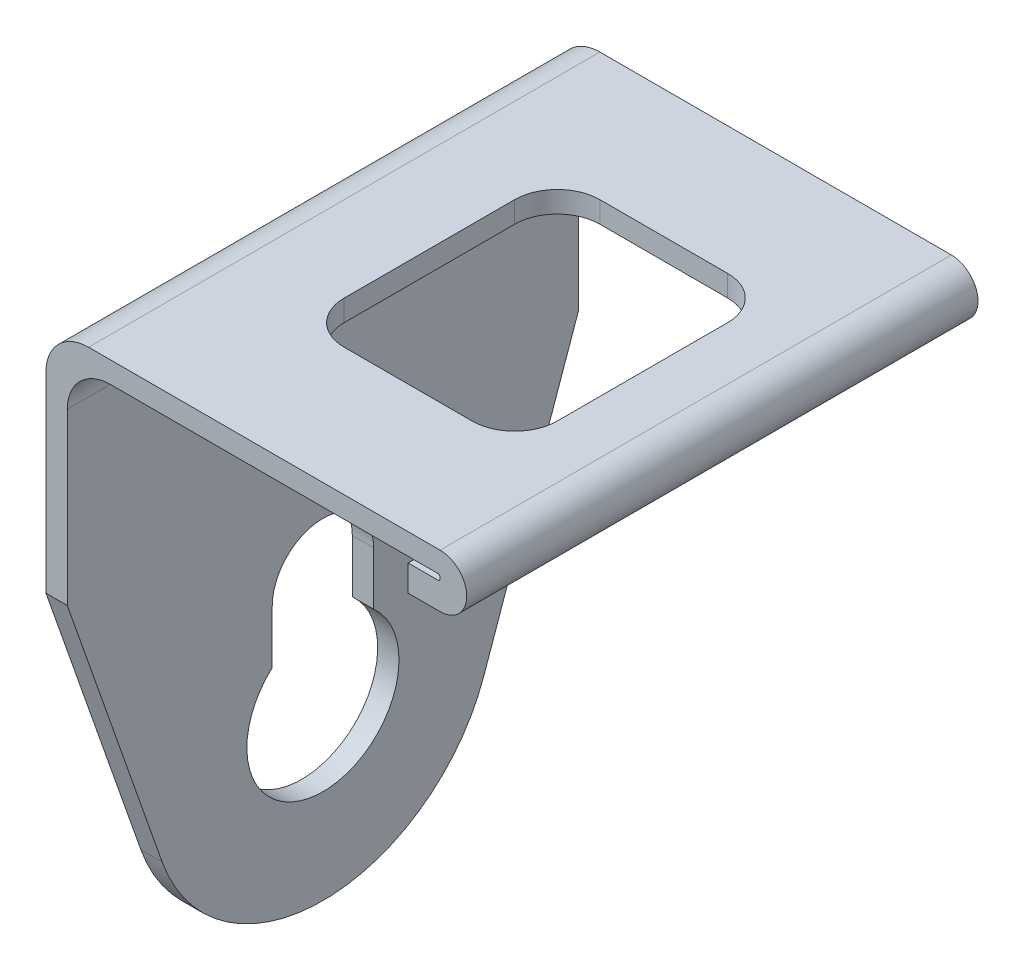
ISO-10303-21;
HEADER;
FILE_DESCRIPTION(('STEP AP214'),'2;1');
FILE_NAME('part.step','',(''),(''),'','','');
FILE_SCHEMA(('AUTOMOTIVE_DESIGN { 1 0 10303 214 1 1 1 1 }'));
ENDSEC;
DATA;
#1=APPLICATION_CONTEXT('core data for automotive mechanical design processes');
#2=APPLICATION_PROTOCOL_DEFINITION('international standard','automotive_design',2000,#1);
#3=PRODUCT_CONTEXT('',#1,'mechanical');
#4=PRODUCT('Part','Part','',(#3));
#5=PRODUCT_RELATED_PRODUCT_CATEGORY('part','',(#4));
#6=PRODUCT_DEFINITION_FORMATION('','',#4);
#7=PRODUCT_DEFINITION_CONTEXT('part definition',#1,'design');
#8=PRODUCT_DEFINITION('design','',#6,#7);
#9=PRODUCT_DEFINITION_SHAPE('','',#8);
#10=(LENGTH_UNIT() NAMED_UNIT(*) SI_UNIT(.MILLI.,.METRE.));
#11=(NAMED_UNIT(*) PLANE_ANGLE_UNIT() SI_UNIT($,.RADIAN.));
#12=(NAMED_UNIT(*) SI_UNIT($,.STERADIAN.) SOLID_ANGLE_UNIT());
#13=UNCERTAINTY_MEASURE_WITH_UNIT(LENGTH_MEASURE(1.E-05),#10,'distance_accuracy_value','');
#14=(GEOMETRIC_REPRESENTATION_CONTEXT(3) GLOBAL_UNCERTAINTY_ASSIGNED_CONTEXT((#13)) GLOBAL_UNIT_ASSIGNED_CONTEXT((#10,
#11,#12)) REPRESENTATION_CONTEXT('',''));
#15=CARTESIAN_POINT('',(0.,0.,0.));
#16=DIRECTION('',(0.,0.,1.));
#17=DIRECTION('',(1.,0.,0.));
#18=AXIS2_PLACEMENT_3D('',#15,#16,#17);
#19=CARTESIAN_POINT('',(0.,-2.,12.));
#20=DIRECTION('',(1.,0.,0.));
#21=DIRECTION('',(0.,1.,0.));
#22=AXIS2_PLACEMENT_3D('',#19,#20,#21);
#23=PLANE('',#22);
#24=DIRECTION('',(0.,1.,0.));
#25=VECTOR('',#24,1.);
#26=CARTESIAN_POINT('',(0.,-2.,-2.38));
#27=LINE('',#26,#25);
#28=CARTESIAN_POINT('',(0.,-18.3390791067752,-2.38));
#29=VERTEX_POINT('',#28);
#30=CARTESIAN_POINT('',(0.,-15.84,-2.38));
#31=VERTEX_POINT('',#30);
#32=EDGE_CURVE('E242',#29,#31,#27,.T.);
#33=ORIENTED_EDGE('',*,*,#32,.T.);
#34=CARTESIAN_POINT('',(0.,-15.84,0.));
#35=DIRECTION('',(1.,0.,0.));
#36=DIRECTION('',(0.,1.,0.));
#37=AXIS2_PLACEMENT_3D('',#34,#35,#36);
#38=CIRCLE('',#37,2.38);
#39=CARTESIAN_POINT('',(0.,-15.84,2.38));
#40=VERTEX_POINT('',#39);
#41=EDGE_CURVE('E245',#31,#40,#38,.T.);
#42=ORIENTED_EDGE('',*,*,#41,.T.);
#43=DIRECTION('',(0.,-1.,0.));
#44=VECTOR('',#43,1.);
#45=CARTESIAN_POINT('',(0.,-2.,2.38));
#46=LINE('',#45,#44);
#47=CARTESIAN_POINT('',(0.,-18.3390791067752,2.38));
#48=VERTEX_POINT('',#47);
#49=EDGE_CURVE('E240',#40,#48,#46,.T.);
#50=ORIENTED_EDGE('',*,*,#49,.T.);
#51=CARTESIAN_POINT('',(0.,-21.,0.));
#52=DIRECTION('',(1.,0.,0.));
#53=DIRECTION('',(0.,1.,0.));
#54=AXIS2_PLACEMENT_3D('',#51,#52,#53);
#55=CIRCLE('',#54,3.57);
#56=EDGE_CURVE('E220',#48,#29,#55,.T.);
#57=ORIENTED_EDGE('',*,*,#56,.T.);
#58=EDGE_LOOP('',(#33,#42,#50,#57));
#59=FACE_BOUND('',#58,.T.);
#60=CARTESIAN_POINT('',(0.,-21.,0.));
#61=DIRECTION('',(1.,0.,0.));
#62=DIRECTION('',(0.,1.,0.));
#63=AXIS2_PLACEMENT_3D('',#60,#61,#62);
#64=CIRCLE('',#63,7.99999999999971);
#65=CARTESIAN_POINT('',(0.,-23.655635881311,7.54636323442549));
#66=VERTEX_POINT('',#65);
#67=CARTESIAN_POINT('',(0.,-23.655635881311,-7.54636323442549));
#68=VERTEX_POINT('',#67);
#69=EDGE_CURVE('E268',#66,#68,#64,.T.);
#70=ORIENTED_EDGE('',*,*,#69,.F.);
#71=DIRECTION('',(0.,-0.943295404303216,-0.331954485163903));
#72=VECTOR('',#71,1.);
#73=CARTESIAN_POINT('',(0.,-2.99174402198394,14.8181802626367));
#74=LINE('',#73,#72);
#75=CARTESIAN_POINT('',(0.,-11.0000000000005,12.));
#76=VERTEX_POINT('',#75);
#77=EDGE_CURVE('E255',#76,#66,#74,.T.);
#78=ORIENTED_EDGE('',*,*,#77,.F.);
#79=DIRECTION('',(0.,-1.,0.));
#80=VECTOR('',#79,1.);
#81=CARTESIAN_POINT('',(0.,-2.,12.));
#82=LINE('',#81,#80);
#83=CARTESIAN_POINT('',(0.,-2.,12.));
#84=VERTEX_POINT('',#83);
#85=EDGE_CURVE('E329',#84,#76,#82,.T.);
#86=ORIENTED_EDGE('',*,*,#85,.F.);
#87=DIRECTION('',(0.,0.,-1.));
#88=VECTOR('',#87,1.);
#89=CARTESIAN_POINT('',(0.,-2.,12.));
#90=LINE('',#89,#88);
#91=CARTESIAN_POINT('',(0.,-2.,-12.));
#92=VERTEX_POINT('',#91);
#93=EDGE_CURVE('E379',#84,#92,#90,.T.);
#94=ORIENTED_EDGE('',*,*,#93,.T.);
#95=DIRECTION('',(0.,-1.,0.));
#96=VECTOR('',#95,1.);
#97=CARTESIAN_POINT('',(0.,-2.,-12.));
#98=LINE('',#97,#96);
#99=CARTESIAN_POINT('',(0.,-11.0000000000005,-12.));
#100=VERTEX_POINT('',#99);
#101=EDGE_CURVE('E353',#92,#100,#98,.T.);
#102=ORIENTED_EDGE('',*,*,#101,.T.);
#103=DIRECTION('',(0.,-0.943295404303216,0.331954485163903));
#104=VECTOR('',#103,1.);
#105=CARTESIAN_POINT('',(0.,-10.5068913890147,-12.1735295373463));
#106=LINE('',#105,#104);
#107=EDGE_CURVE('E264',#100,#68,#106,.T.);
#108=ORIENTED_EDGE('',*,*,#107,.T.);
#109=EDGE_LOOP('',(#70,#78,#86,#94,#102,#108));
#110=FACE_BOUND('',#109,.T.);
#111=ADVANCED_FACE('F39',(#59,#110),#23,.F.);
#112=CARTESIAN_POINT('',(1.,-29.,12.));
#113=DIRECTION('',(-1.,0.,0.));
#114=DIRECTION('',(0.,-1.,0.));
#115=AXIS2_PLACEMENT_3D('',#112,#113,#114);
#116=PLANE('',#115);
#117=DIRECTION('',(0.,-1.,0.));
#118=VECTOR('',#117,1.);
#119=CARTESIAN_POINT('',(1.,-15.84,2.38));
#120=LINE('',#119,#118);
#121=CARTESIAN_POINT('',(1.,-15.84,2.38));
#122=VERTEX_POINT('',#121);
#123=CARTESIAN_POINT('',(1.,-18.3390791067752,2.38));
#124=VERTEX_POINT('',#123);
#125=EDGE_CURVE('E224',#122,#124,#120,.T.);
#126=ORIENTED_EDGE('',*,*,#125,.F.);
#127=CARTESIAN_POINT('',(1.,-15.84,0.));
#128=DIRECTION('',(1.,0.,0.));
#129=DIRECTION('',(0.,1.,0.));
#130=AXIS2_PLACEMENT_3D('',#127,#128,#129);
#131=CIRCLE('',#130,2.38);
#132=CARTESIAN_POINT('',(1.,-15.84,-2.38));
#133=VERTEX_POINT('',#132);
#134=EDGE_CURVE('E62',#133,#122,#131,.T.);
#135=ORIENTED_EDGE('',*,*,#134,.F.);
#136=DIRECTION('',(0.,1.,0.));
#137=VECTOR('',#136,1.);
#138=CARTESIAN_POINT('',(1.,-15.84,-2.38));
#139=LINE('',#138,#137);
#140=CARTESIAN_POINT('',(1.,-18.3390791067752,-2.38));
#141=VERTEX_POINT('',#140);
#142=EDGE_CURVE('E230',#141,#133,#139,.T.);
#143=ORIENTED_EDGE('',*,*,#142,.F.);
#144=CARTESIAN_POINT('',(1.,-21.,0.));
#145=DIRECTION('',(1.,0.,0.));
#146=DIRECTION('',(0.,1.,0.));
#147=AXIS2_PLACEMENT_3D('',#144,#145,#146);
#148=CIRCLE('',#147,3.57);
#149=EDGE_CURVE('E212',#124,#141,#148,.T.);
#150=ORIENTED_EDGE('',*,*,#149,.F.);
#151=EDGE_LOOP('',(#126,#135,#143,#150));
#152=FACE_BOUND('',#151,.T.);
#153=DIRECTION('',(0.,-0.943295404303216,-0.331954485163903));
#154=VECTOR('',#153,1.);
#155=CARTESIAN_POINT('',(1.,-4.96970526594021,14.1221171805774));
#156=LINE('',#155,#154);
#157=CARTESIAN_POINT('',(1.,-11.0000000000005,12.));
#158=VERTEX_POINT('',#157);
#159=CARTESIAN_POINT('',(1.,-23.655635881311,7.54636323442549));
#160=VERTEX_POINT('',#159);
#161=EDGE_CURVE('E247',#158,#160,#156,.T.);
#162=ORIENTED_EDGE('',*,*,#161,.T.);
#163=CARTESIAN_POINT('',(1.,-21.,0.));
#164=DIRECTION('',(1.,0.,0.));
#165=DIRECTION('',(0.,1.,0.));
#166=AXIS2_PLACEMENT_3D('',#163,#164,#165);
#167=CIRCLE('',#166,7.99999999999971);
#168=CARTESIAN_POINT('',(1.,-23.655635881311,-7.54636323442549));
#169=VERTEX_POINT('',#168);
#170=EDGE_CURVE('E260',#160,#169,#167,.T.);
#171=ORIENTED_EDGE('',*,*,#170,.T.);
#172=DIRECTION('',(0.,-0.943295404303216,0.331954485163903));
#173=VECTOR('',#172,1.);
#174=CARTESIAN_POINT('',(1.,-4.9697052659402,-14.1221171805774));
#175=LINE('',#174,#173);
#176=CARTESIAN_POINT('',(1.,-11.0000000000004,-12.));
#177=VERTEX_POINT('',#176);
#178=EDGE_CURVE('E257',#177,#169,#175,.T.);
#179=ORIENTED_EDGE('',*,*,#178,.F.);
#180=DIRECTION('',(0.,1.,0.));
#181=VECTOR('',#180,1.);
#182=CARTESIAN_POINT('',(1.,-29.,-12.));
#183=LINE('',#182,#181);
#184=CARTESIAN_POINT('',(1.,-3.02138494167755,-12.));
#185=VERTEX_POINT('',#184);
#186=EDGE_CURVE('E359',#177,#185,#183,.T.);
#187=ORIENTED_EDGE('',*,*,#186,.T.);
#188=DIRECTION('',(0.,0.,-1.));
#189=VECTOR('',#188,1.);
#190=CARTESIAN_POINT('',(1.,-3.02138494167755,12.));
#191=LINE('',#190,#189);
#192=CARTESIAN_POINT('',(1.,-3.02138494167755,12.));
#193=VERTEX_POINT('',#192);
#194=EDGE_CURVE('E380',#193,#185,#191,.T.);
#195=ORIENTED_EDGE('',*,*,#194,.F.);
#196=DIRECTION('',(0.,1.,0.));
#197=VECTOR('',#196,1.);
#198=CARTESIAN_POINT('',(1.,-29.,12.));
#199=LINE('',#198,#197);
#200=EDGE_CURVE('E334',#158,#193,#199,.T.);
#201=ORIENTED_EDGE('',*,*,#200,.F.);
#202=EDGE_LOOP('',(#162,#171,#179,#187,#195,#201));
#203=FACE_BOUND('',#202,.T.);
#204=ADVANCED_FACE('F227',(#152,#203),#116,.F.);
#205=CARTESIAN_POINT('',(18.3072028533605,-1.13435028841984,12.));
#206=DIRECTION('',(0.,0.,-1.));
#207=DIRECTION('',(-1.,0.,0.));
#208=AXIS2_PLACEMENT_3D('',#205,#206,#207);
#209=PLANE('',#208);
#210=DIRECTION('',(-1.,0.,0.));
#211=VECTOR('',#210,1.);
#212=CARTESIAN_POINT('',(18.3072028533605,-11.0000000000004,12.));
#213=LINE('',#212,#211);
#214=EDGE_CURVE('E11',#158,#76,#213,.T.);
#215=ORIENTED_EDGE('',*,*,#214,.F.);
#216=ORIENTED_EDGE('',*,*,#200,.T.);
#217=CARTESIAN_POINT('',(3.02138494167756,-3.02138494167755,12.));
#218=DIRECTION('',(0.,0.,-1.));
#219=DIRECTION('',(1.,0.,0.));
#220=AXIS2_PLACEMENT_3D('',#217,#218,#219);
#221=CIRCLE('',#220,2.02138494167755);
#222=CARTESIAN_POINT('',(3.02138494167756,-1.,12.));
#223=VERTEX_POINT('',#222);
#224=EDGE_CURVE('E333',#193,#223,#221,.T.);
#225=ORIENTED_EDGE('',*,*,#224,.T.);
#226=DIRECTION('',(1.,0.,0.));
#227=VECTOR('',#226,1.);
#228=CARTESIAN_POINT('',(3.02138494167756,-1.,12.));
#229=LINE('',#228,#227);
#230=CARTESIAN_POINT('',(18.4415531417916,-1.,12.));
#231=VERTEX_POINT('',#230);
#232=EDGE_CURVE('E337',#223,#231,#229,.T.);
#233=ORIENTED_EDGE('',*,*,#232,.T.);
#234=CARTESIAN_POINT('',(18.3072028533605,-1.13435028841984,12.));
#235=DIRECTION('',(0.,0.,-1.));
#236=DIRECTION('',(-1.,0.,0.));
#237=AXIS2_PLACEMENT_3D('',#234,#235,#236);
#238=CIRCLE('',#237,0.19);
#239=CARTESIAN_POINT('',(18.4415531417916,-1.26870057683967,12.));
#240=VERTEX_POINT('',#239);
#241=EDGE_CURVE('E338',#231,#240,#238,.T.);
#242=ORIENTED_EDGE('',*,*,#241,.T.);
#243=DIRECTION('',(-1.,0.,0.));
#244=VECTOR('',#243,1.);
#245=CARTESIAN_POINT('',(18.4415531417916,-1.26870057683967,12.));
#246=LINE('',#245,#244);
#247=CARTESIAN_POINT('',(17.,-1.26870057683967,12.));
#248=VERTEX_POINT('',#247);
#249=EDGE_CURVE('E343',#240,#248,#246,.T.);
#250=ORIENTED_EDGE('',*,*,#249,.T.);
#251=DIRECTION('',(0.,-1.,0.));
#252=VECTOR('',#251,1.);
#253=CARTESIAN_POINT('',(17.,-2.5,12.));
#254=LINE('',#253,#252);
#255=CARTESIAN_POINT('',(17.,-2.5,12.));
#256=VERTEX_POINT('',#255);
#257=EDGE_CURVE('E318',#248,#256,#254,.T.);
#258=ORIENTED_EDGE('',*,*,#257,.T.);
#259=DIRECTION('',(1.,0.,0.));
#260=VECTOR('',#259,1.);
#261=CARTESIAN_POINT('',(18.5,-2.5,12.));
#262=LINE('',#261,#260);
#263=CARTESIAN_POINT('',(18.5,-2.5,12.));
#264=VERTEX_POINT('',#263);
#265=EDGE_CURVE('E321',#256,#264,#262,.T.);
#266=ORIENTED_EDGE('',*,*,#265,.T.);
#267=CARTESIAN_POINT('',(18.5,-1.25,12.));
#268=DIRECTION('',(0.,0.,1.));
#269=DIRECTION('',(1.,0.,0.));
#270=AXIS2_PLACEMENT_3D('',#267,#268,#269);
#271=CIRCLE('',#270,1.25);
#272=CARTESIAN_POINT('',(18.5,0.,12.));
#273=VERTEX_POINT('',#272);
#274=EDGE_CURVE('E322',#264,#273,#271,.T.);
#275=ORIENTED_EDGE('',*,*,#274,.T.);
#276=DIRECTION('',(-1.,0.,0.));
#277=VECTOR('',#276,1.);
#278=CARTESIAN_POINT('',(2.,0.,12.));
#279=LINE('',#278,#277);
#280=CARTESIAN_POINT('',(2.,0.,12.));
#281=VERTEX_POINT('',#280);
#282=EDGE_CURVE('E326',#273,#281,#279,.T.);
#283=ORIENTED_EDGE('',*,*,#282,.T.);
#284=CARTESIAN_POINT('',(2.,-2.,12.));
#285=DIRECTION('',(0.,0.,1.));
#286=DIRECTION('',(1.,0.,0.));
#287=AXIS2_PLACEMENT_3D('',#284,#285,#286);
#288=CIRCLE('',#287,2.);
#289=EDGE_CURVE('E327',#281,#84,#288,.T.);
#290=ORIENTED_EDGE('',*,*,#289,.T.);
#291=ORIENTED_EDGE('',*,*,#85,.T.);
#292=EDGE_LOOP('',(#215,#216,#225,#233,#242,#250,#258,#266,#275,#283,#290,#291));
#293=FACE_BOUND('',#292,.T.);
#294=ADVANCED_FACE('F445',(#293),#209,.F.);
#295=CARTESIAN_POINT('',(17.,-2.5,12.));
#296=DIRECTION('',(1.,0.,0.));
#297=DIRECTION('',(0.,0.,-1.));
#298=AXIS2_PLACEMENT_3D('',#295,#296,#297);
#299=PLANE('',#298);
#300=DIRECTION('',(0.,-1.,0.));
#301=VECTOR('',#300,1.);
#302=CARTESIAN_POINT('',(17.,-2.5,-12.));
#303=LINE('',#302,#301);
#304=CARTESIAN_POINT('',(17.,-1.26870057683967,-12.));
#305=VERTEX_POINT('',#304);
#306=CARTESIAN_POINT('',(17.,-2.5,-12.));
#307=VERTEX_POINT('',#306);
#308=EDGE_CURVE('E320',#305,#307,#303,.T.);
#309=ORIENTED_EDGE('',*,*,#308,.T.);
#310=DIRECTION('',(0.,0.,-1.));
#311=VECTOR('',#310,1.);
#312=CARTESIAN_POINT('',(17.,-2.5,12.));
#313=LINE('',#312,#311);
#314=EDGE_CURVE('E392',#256,#307,#313,.T.);
#315=ORIENTED_EDGE('',*,*,#314,.F.);
#316=ORIENTED_EDGE('',*,*,#257,.F.);
#317=DIRECTION('',(0.,0.,-1.));
#318=VECTOR('',#317,1.);
#319=CARTESIAN_POINT('',(17.,-1.26870057683967,12.));
#320=LINE('',#319,#318);
#321=EDGE_CURVE('E342',#248,#305,#320,.T.);
#322=ORIENTED_EDGE('',*,*,#321,.T.);
#323=EDGE_LOOP('',(#309,#315,#316,#322));
#324=FACE_BOUND('',#323,.T.);
#325=ADVANCED_FACE('F41',(#324),#299,.F.);
#326=CARTESIAN_POINT('',(18.5,-2.5,12.));
#327=DIRECTION('',(0.,1.,0.));
#328=DIRECTION('',(0.,0.,1.));
#329=AXIS2_PLACEMENT_3D('',#326,#327,#328);
#330=PLANE('',#329);
#331=DIRECTION('',(1.,0.,0.));
#332=VECTOR('',#331,1.);
#333=CARTESIAN_POINT('',(18.5,-2.5,-12.));
#334=LINE('',#333,#332);
#335=CARTESIAN_POINT('',(18.5,-2.5,-12.));
#336=VERTEX_POINT('',#335);
#337=EDGE_CURVE('E347',#307,#336,#334,.T.);
#338=ORIENTED_EDGE('',*,*,#337,.T.);
#339=DIRECTION('',(0.,0.,-1.));
#340=VECTOR('',#339,1.);
#341=CARTESIAN_POINT('',(18.5,-2.5,12.));
#342=LINE('',#341,#340);
#343=EDGE_CURVE('E386',#264,#336,#342,.T.);
#344=ORIENTED_EDGE('',*,*,#343,.F.);
#345=ORIENTED_EDGE('',*,*,#265,.F.);
#346=ORIENTED_EDGE('',*,*,#314,.T.);
#347=EDGE_LOOP('',(#338,#344,#345,#346));
#348=FACE_BOUND('',#347,.T.);
#349=ADVANCED_FACE('F471',(#348),#330,.F.);
#350=CARTESIAN_POINT('',(18.5,-1.25,12.));
#351=DIRECTION('',(0.,0.,-1.));
#352=DIRECTION('',(-1.,0.,0.));
#353=AXIS2_PLACEMENT_3D('',#350,#351,#352);
#354=CYLINDRICAL_SURFACE('',#353,1.25);
#355=CARTESIAN_POINT('',(18.5,-1.25,-12.));
#356=DIRECTION('',(0.,0.,1.));
#357=DIRECTION('',(1.,0.,0.));
#358=AXIS2_PLACEMENT_3D('',#355,#356,#357);
#359=CIRCLE('',#358,1.25);
#360=CARTESIAN_POINT('',(18.5,0.,-12.));
#361=VERTEX_POINT('',#360);
#362=EDGE_CURVE('E346',#336,#361,#359,.T.);
#363=ORIENTED_EDGE('',*,*,#362,.T.);
#364=DIRECTION('',(0.,0.,-1.));
#365=VECTOR('',#364,1.);
#366=CARTESIAN_POINT('',(18.5,0.,12.));
#367=LINE('',#366,#365);
#368=EDGE_CURVE('E387',#273,#361,#367,.T.);
#369=ORIENTED_EDGE('',*,*,#368,.F.);
#370=ORIENTED_EDGE('',*,*,#274,.F.);
#371=ORIENTED_EDGE('',*,*,#343,.T.);
#372=EDGE_LOOP('',(#363,#369,#370,#371));
#373=FACE_BOUND('',#372,.T.);
#374=ADVANCED_FACE('F469',(#373),#354,.T.);
#375=CARTESIAN_POINT('',(2.,0.,12.));
#376=DIRECTION('',(0.,-1.,0.));
#377=DIRECTION('',(0.,0.,-1.));
#378=AXIS2_PLACEMENT_3D('',#375,#376,#377);
#379=PLANE('',#378);
#380=DIRECTION('',(0.,0.,1.));
#381=VECTOR('',#380,1.);
#382=CARTESIAN_POINT('',(16.,0.,12.));
#383=LINE('',#382,#381);
#384=CARTESIAN_POINT('',(16.,0.,-4.));
#385=VERTEX_POINT('',#384);
#386=CARTESIAN_POINT('',(16.,0.,4.));
#387=VERTEX_POINT('',#386);
#388=EDGE_CURVE('E313',#385,#387,#383,.T.);
#389=ORIENTED_EDGE('',*,*,#388,.T.);
#390=CARTESIAN_POINT('',(14.,0.,4.));
#391=DIRECTION('',(0.,-1.,0.));
#392=DIRECTION('',(0.,0.,-1.));
#393=AXIS2_PLACEMENT_3D('',#390,#391,#392);
#394=CIRCLE('',#393,2.);
#395=CARTESIAN_POINT('',(14.,0.,6.));
#396=VERTEX_POINT('',#395);
#397=EDGE_CURVE('E314',#387,#396,#394,.T.);
#398=ORIENTED_EDGE('',*,*,#397,.T.);
#399=DIRECTION('',(-1.,0.,0.));
#400=VECTOR('',#399,1.);
#401=CARTESIAN_POINT('',(2.,0.,6.));
#402=LINE('',#401,#400);
#403=CARTESIAN_POINT('',(8.,0.,6.));
#404=VERTEX_POINT('',#403);
#405=EDGE_CURVE('E273',#396,#404,#402,.T.);
#406=ORIENTED_EDGE('',*,*,#405,.T.);
#407=CARTESIAN_POINT('',(8.,0.,4.));
#408=DIRECTION('',(0.,-1.,0.));
#409=DIRECTION('',(0.,0.,-1.));
#410=AXIS2_PLACEMENT_3D('',#407,#408,#409);
#411=CIRCLE('',#410,2.);
#412=CARTESIAN_POINT('',(6.,0.,4.));
#413=VERTEX_POINT('',#412);
#414=EDGE_CURVE('E296',#404,#413,#411,.T.);
#415=ORIENTED_EDGE('',*,*,#414,.T.);
#416=DIRECTION('',(0.,0.,-1.));
#417=VECTOR('',#416,1.);
#418=CARTESIAN_POINT('',(6.,0.,12.));
#419=LINE('',#418,#417);
#420=CARTESIAN_POINT('',(6.,0.,-4.));
#421=VERTEX_POINT('',#420);
#422=EDGE_CURVE('E298',#413,#421,#419,.T.);
#423=ORIENTED_EDGE('',*,*,#422,.T.);
#424=CARTESIAN_POINT('',(8.,0.,-4.));
#425=DIRECTION('',(0.,-1.,0.));
#426=DIRECTION('',(0.,0.,-1.));
#427=AXIS2_PLACEMENT_3D('',#424,#425,#426);
#428=CIRCLE('',#427,2.);
#429=CARTESIAN_POINT('',(8.,0.,-6.));
#430=VERTEX_POINT('',#429);
#431=EDGE_CURVE('E304',#421,#430,#428,.T.);
#432=ORIENTED_EDGE('',*,*,#431,.T.);
#433=DIRECTION('',(1.,0.,0.));
#434=VECTOR('',#433,1.);
#435=CARTESIAN_POINT('',(2.,0.,-6.));
#436=LINE('',#435,#434);
#437=CARTESIAN_POINT('',(14.,0.,-6.));
#438=VERTEX_POINT('',#437);
#439=EDGE_CURVE('E301',#430,#438,#436,.T.);
#440=ORIENTED_EDGE('',*,*,#439,.T.);
#441=CARTESIAN_POINT('',(14.,0.,-4.));
#442=DIRECTION('',(0.,-1.,0.));
#443=DIRECTION('',(0.,0.,-1.));
#444=AXIS2_PLACEMENT_3D('',#441,#442,#443);
#445=CIRCLE('',#444,2.);
#446=EDGE_CURVE('E306',#438,#385,#445,.T.);
#447=ORIENTED_EDGE('',*,*,#446,.T.);
#448=EDGE_LOOP('',(#389,#398,#406,#415,#423,#432,#440,#447));
#449=FACE_BOUND('',#448,.T.);
#450=DIRECTION('',(-1.,0.,0.));
#451=VECTOR('',#450,1.);
#452=CARTESIAN_POINT('',(2.,0.,-12.));
#453=LINE('',#452,#451);
#454=CARTESIAN_POINT('',(2.,0.,-12.));
#455=VERTEX_POINT('',#454);
#456=EDGE_CURVE('E348',#361,#455,#453,.T.);
#457=ORIENTED_EDGE('',*,*,#456,.T.);
#458=DIRECTION('',(0.,0.,-1.));
#459=VECTOR('',#458,1.);
#460=CARTESIAN_POINT('',(2.,0.,12.));
#461=LINE('',#460,#459);
#462=EDGE_CURVE('E382',#281,#455,#461,.T.);
#463=ORIENTED_EDGE('',*,*,#462,.F.);
#464=ORIENTED_EDGE('',*,*,#282,.F.);
#465=ORIENTED_EDGE('',*,*,#368,.T.);
#466=EDGE_LOOP('',(#457,#463,#464,#465));
#467=FACE_BOUND('',#466,.T.);
#468=ADVANCED_FACE('F464',(#449,#467),#379,.F.);
#469=CARTESIAN_POINT('',(2.,-2.,12.));
#470=DIRECTION('',(0.,0.,-1.));
#471=DIRECTION('',(-1.,0.,0.));
#472=AXIS2_PLACEMENT_3D('',#469,#470,#471);
#473=CYLINDRICAL_SURFACE('',#472,2.);
#474=CARTESIAN_POINT('',(2.,-2.,-12.));
#475=DIRECTION('',(0.,0.,1.));
#476=DIRECTION('',(1.,0.,0.));
#477=AXIS2_PLACEMENT_3D('',#474,#475,#476);
#478=CIRCLE('',#477,2.);
#479=EDGE_CURVE('E352',#455,#92,#478,.T.);
#480=ORIENTED_EDGE('',*,*,#479,.T.);
#481=ORIENTED_EDGE('',*,*,#93,.F.);
#482=ORIENTED_EDGE('',*,*,#289,.F.);
#483=ORIENTED_EDGE('',*,*,#462,.T.);
#484=EDGE_LOOP('',(#480,#481,#482,#483));
#485=FACE_BOUND('',#484,.T.);
#486=ADVANCED_FACE('F456',(#485),#473,.T.);
#487=CARTESIAN_POINT('',(3.02138494167756,-3.02138494167755,12.));
#488=DIRECTION('',(0.,0.,-1.));
#489=DIRECTION('',(-1.,0.,0.));
#490=AXIS2_PLACEMENT_3D('',#487,#488,#489);
#491=CYLINDRICAL_SURFACE('',#490,2.02138494167755);
#492=CARTESIAN_POINT('',(3.02138494167756,-3.02138494167755,-12.));
#493=DIRECTION('',(0.,0.,-1.));
#494=DIRECTION('',(1.,0.,0.));
#495=AXIS2_PLACEMENT_3D('',#492,#493,#494);
#496=CIRCLE('',#495,2.02138494167755);
#497=CARTESIAN_POINT('',(3.02138494167756,-1.,-12.));
#498=VERTEX_POINT('',#497);
#499=EDGE_CURVE('E360',#185,#498,#496,.T.);
#500=ORIENTED_EDGE('',*,*,#499,.T.);
#501=DIRECTION('',(0.,0.,-1.));
#502=VECTOR('',#501,1.);
#503=CARTESIAN_POINT('',(3.02138494167756,-1.,12.));
#504=LINE('',#503,#502);
#505=EDGE_CURVE('E372',#223,#498,#504,.T.);
#506=ORIENTED_EDGE('',*,*,#505,.F.);
#507=ORIENTED_EDGE('',*,*,#224,.F.);
#508=ORIENTED_EDGE('',*,*,#194,.T.);
#509=EDGE_LOOP('',(#500,#506,#507,#508));
#510=FACE_BOUND('',#509,.T.);
#511=ADVANCED_FACE('F433',(#510),#491,.F.);
#512=CARTESIAN_POINT('',(3.02138494167756,-1.,12.));
#513=DIRECTION('',(0.,1.,0.));
#514=DIRECTION('',(0.,0.,1.));
#515=AXIS2_PLACEMENT_3D('',#512,#513,#514);
#516=PLANE('',#515);
#517=DIRECTION('',(1.,0.,0.));
#518=VECTOR('',#517,1.);
#519=CARTESIAN_POINT('',(3.02138494167755,-1.,6.));
#520=LINE('',#519,#518);
#521=CARTESIAN_POINT('',(8.,-1.,6.));
#522=VERTEX_POINT('',#521);
#523=CARTESIAN_POINT('',(14.,-1.,6.));
#524=VERTEX_POINT('',#523);
#525=EDGE_CURVE('E395',#522,#524,#520,.T.);
#526=ORIENTED_EDGE('',*,*,#525,.T.);
#527=CARTESIAN_POINT('',(14.,-1.,4.));
#528=DIRECTION('',(0.,1.,0.));
#529=DIRECTION('',(0.,0.,1.));
#530=AXIS2_PLACEMENT_3D('',#527,#528,#529);
#531=CIRCLE('',#530,2.);
#532=CARTESIAN_POINT('',(16.,-1.,4.));
#533=VERTEX_POINT('',#532);
#534=EDGE_CURVE('E418',#524,#533,#531,.T.);
#535=ORIENTED_EDGE('',*,*,#534,.T.);
#536=DIRECTION('',(0.,0.,-1.));
#537=VECTOR('',#536,1.);
#538=CARTESIAN_POINT('',(16.,-1.,12.));
#539=LINE('',#538,#537);
#540=CARTESIAN_POINT('',(16.,-1.,-4.));
#541=VERTEX_POINT('',#540);
#542=EDGE_CURVE('E412',#533,#541,#539,.T.);
#543=ORIENTED_EDGE('',*,*,#542,.T.);
#544=CARTESIAN_POINT('',(14.,-1.,-4.));
#545=DIRECTION('',(0.,1.,0.));
#546=DIRECTION('',(0.,0.,1.));
#547=AXIS2_PLACEMENT_3D('',#544,#545,#546);
#548=CIRCLE('',#547,2.);
#549=CARTESIAN_POINT('',(14.,-1.,-6.));
#550=VERTEX_POINT('',#549);
#551=EDGE_CURVE('E410',#541,#550,#548,.T.);
#552=ORIENTED_EDGE('',*,*,#551,.T.);
#553=DIRECTION('',(-1.,0.,0.));
#554=VECTOR('',#553,1.);
#555=CARTESIAN_POINT('',(3.02138494167756,-1.,-6.));
#556=LINE('',#555,#554);
#557=CARTESIAN_POINT('',(8.,-1.,-6.));
#558=VERTEX_POINT('',#557);
#559=EDGE_CURVE('E407',#550,#558,#556,.T.);
#560=ORIENTED_EDGE('',*,*,#559,.T.);
#561=CARTESIAN_POINT('',(8.,-1.,-4.));
#562=DIRECTION('',(0.,1.,0.));
#563=DIRECTION('',(0.,0.,1.));
#564=AXIS2_PLACEMENT_3D('',#561,#562,#563);
#565=CIRCLE('',#564,2.);
#566=CARTESIAN_POINT('',(6.,-1.,-4.));
#567=VERTEX_POINT('',#566);
#568=EDGE_CURVE('E404',#558,#567,#565,.T.);
#569=ORIENTED_EDGE('',*,*,#568,.T.);
#570=DIRECTION('',(0.,0.,1.));
#571=VECTOR('',#570,1.);
#572=CARTESIAN_POINT('',(6.,-1.,12.));
#573=LINE('',#572,#571);
#574=CARTESIAN_POINT('',(6.,-1.,4.));
#575=VERTEX_POINT('',#574);
#576=EDGE_CURVE('E402',#567,#575,#573,.T.);
#577=ORIENTED_EDGE('',*,*,#576,.T.);
#578=CARTESIAN_POINT('',(8.,-1.,4.));
#579=DIRECTION('',(0.,1.,0.));
#580=DIRECTION('',(0.,0.,1.));
#581=AXIS2_PLACEMENT_3D('',#578,#579,#580);
#582=CIRCLE('',#581,2.);
#583=EDGE_CURVE('E397',#575,#522,#582,.T.);
#584=ORIENTED_EDGE('',*,*,#583,.T.);
#585=EDGE_LOOP('',(#526,#535,#543,#552,#560,#569,#577,#584));
#586=FACE_BOUND('',#585,.T.);
#587=DIRECTION('',(1.,0.,0.));
#588=VECTOR('',#587,1.);
#589=CARTESIAN_POINT('',(3.02138494167756,-1.,-12.));
#590=LINE('',#589,#588);
#591=CARTESIAN_POINT('',(18.4415531417916,-1.,-12.));
#592=VERTEX_POINT('',#591);
#593=EDGE_CURVE('E363',#498,#592,#590,.T.);
#594=ORIENTED_EDGE('',*,*,#593,.T.);
#595=DIRECTION('',(0.,0.,-1.));
#596=VECTOR('',#595,1.);
#597=CARTESIAN_POINT('',(18.4415531417916,-1.,12.));
#598=LINE('',#597,#596);
#599=EDGE_CURVE('E371',#231,#592,#598,.T.);
#600=ORIENTED_EDGE('',*,*,#599,.F.);
#601=ORIENTED_EDGE('',*,*,#232,.F.);
#602=ORIENTED_EDGE('',*,*,#505,.T.);
#603=EDGE_LOOP('',(#594,#600,#601,#602));
#604=FACE_BOUND('',#603,.T.);
#605=ADVANCED_FACE('F440',(#586,#604),#516,.F.);
#606=CARTESIAN_POINT('',(18.3072028533605,-1.13435028841984,12.));
#607=DIRECTION('',(0.,0.,-1.));
#608=DIRECTION('',(-1.,0.,0.));
#609=AXIS2_PLACEMENT_3D('',#606,#607,#608);
#610=CYLINDRICAL_SURFACE('',#609,0.19);
#611=CARTESIAN_POINT('',(18.3072028533605,-1.13435028841984,-12.));
#612=DIRECTION('',(0.,0.,-1.));
#613=DIRECTION('',(-1.,0.,0.));
#614=AXIS2_PLACEMENT_3D('',#611,#612,#613);
#615=CIRCLE('',#614,0.19);
#616=CARTESIAN_POINT('',(18.4415531417916,-1.26870057683967,-12.));
#617=VERTEX_POINT('',#616);
#618=EDGE_CURVE('E361',#592,#617,#615,.T.);
#619=ORIENTED_EDGE('',*,*,#618,.T.);
#620=DIRECTION('',(0.,0.,-1.));
#621=VECTOR('',#620,1.);
#622=CARTESIAN_POINT('',(18.4415531417916,-1.26870057683967,12.));
#623=LINE('',#622,#621);
#624=EDGE_CURVE('E366',#240,#617,#623,.T.);
#625=ORIENTED_EDGE('',*,*,#624,.F.);
#626=ORIENTED_EDGE('',*,*,#241,.F.);
#627=ORIENTED_EDGE('',*,*,#599,.T.);
#628=EDGE_LOOP('',(#619,#625,#626,#627));
#629=FACE_BOUND('',#628,.T.);
#630=ADVANCED_FACE('F481',(#629),#610,.F.);
#631=CARTESIAN_POINT('',(18.4415531417916,-1.26870057683967,12.));
#632=DIRECTION('',(0.,-1.,0.));
#633=DIRECTION('',(1.,0.,0.));
#634=AXIS2_PLACEMENT_3D('',#631,#632,#633);
#635=PLANE('',#634);
#636=DIRECTION('',(-1.,0.,0.));
#637=VECTOR('',#636,1.);
#638=CARTESIAN_POINT('',(18.4415531417916,-1.26870057683967,-12.));
#639=LINE('',#638,#637);
#640=EDGE_CURVE('E325',#617,#305,#639,.T.);
#641=ORIENTED_EDGE('',*,*,#640,.T.);
#642=ORIENTED_EDGE('',*,*,#321,.F.);
#643=ORIENTED_EDGE('',*,*,#249,.F.);
#644=ORIENTED_EDGE('',*,*,#624,.T.);
#645=EDGE_LOOP('',(#641,#642,#643,#644));
#646=FACE_BOUND('',#645,.T.);
#647=ADVANCED_FACE('F479',(#646),#635,.F.);
#648=CARTESIAN_POINT('',(18.3072028533605,-1.13435028841984,-12.));
#649=DIRECTION('',(0.,0.,-1.));
#650=DIRECTION('',(-1.,0.,0.));
#651=AXIS2_PLACEMENT_3D('',#648,#649,#650);
#652=PLANE('',#651);
#653=DIRECTION('',(1.,0.,0.));
#654=VECTOR('',#653,1.);
#655=CARTESIAN_POINT('',(18.3072028533605,-11.0000000000005,-12.));
#656=LINE('',#655,#654);
#657=EDGE_CURVE('E50',#100,#177,#656,.T.);
#658=ORIENTED_EDGE('',*,*,#657,.F.);
#659=ORIENTED_EDGE('',*,*,#101,.F.);
#660=ORIENTED_EDGE('',*,*,#479,.F.);
#661=ORIENTED_EDGE('',*,*,#456,.F.);
#662=ORIENTED_EDGE('',*,*,#362,.F.);
#663=ORIENTED_EDGE('',*,*,#337,.F.);
#664=ORIENTED_EDGE('',*,*,#308,.F.);
#665=ORIENTED_EDGE('',*,*,#640,.F.);
#666=ORIENTED_EDGE('',*,*,#618,.F.);
#667=ORIENTED_EDGE('',*,*,#593,.F.);
#668=ORIENTED_EDGE('',*,*,#499,.F.);
#669=ORIENTED_EDGE('',*,*,#186,.F.);
#670=EDGE_LOOP('',(#658,#659,#660,#661,#662,#663,#664,#665,#666,#667,#668,#669));
#671=FACE_BOUND('',#670,.T.);
#672=ADVANCED_FACE('F428',(#671),#652,.T.);
#673=CARTESIAN_POINT('',(14.,4.,4.));
#674=DIRECTION('',(0.,-1.,0.));
#675=DIRECTION('',(0.,0.,-1.));
#676=AXIS2_PLACEMENT_3D('',#673,#674,#675);
#677=CYLINDRICAL_SURFACE('',#676,2.);
#678=DIRECTION('',(0.,-1.,0.));
#679=VECTOR('',#678,1.);
#680=CARTESIAN_POINT('',(16.,4.,4.));
#681=LINE('',#680,#679);
#682=EDGE_CURVE('E271',#387,#533,#681,.T.);
#683=ORIENTED_EDGE('',*,*,#682,.T.);
#684=ORIENTED_EDGE('',*,*,#534,.F.);
#685=DIRECTION('',(0.,-1.,0.));
#686=VECTOR('',#685,1.);
#687=CARTESIAN_POINT('',(14.,4.,6.));
#688=LINE('',#687,#686);
#689=EDGE_CURVE('E269',#396,#524,#688,.T.);
#690=ORIENTED_EDGE('',*,*,#689,.F.);
#691=ORIENTED_EDGE('',*,*,#397,.F.);
#692=EDGE_LOOP('',(#683,#684,#690,#691));
#693=FACE_BOUND('',#692,.T.);
#694=ADVANCED_FACE('F524',(#693),#677,.F.);
#695=CARTESIAN_POINT('',(16.,4.,4.));
#696=DIRECTION('',(1.,0.,0.));
#697=DIRECTION('',(0.,0.,-1.));
#698=AXIS2_PLACEMENT_3D('',#695,#696,#697);
#699=PLANE('',#698);
#700=DIRECTION('',(0.,-1.,0.));
#701=VECTOR('',#700,1.);
#702=CARTESIAN_POINT('',(16.,4.,-4.));
#703=LINE('',#702,#701);
#704=EDGE_CURVE('E274',#385,#541,#703,.T.);
#705=ORIENTED_EDGE('',*,*,#704,.T.);
#706=ORIENTED_EDGE('',*,*,#542,.F.);
#707=ORIENTED_EDGE('',*,*,#682,.F.);
#708=ORIENTED_EDGE('',*,*,#388,.F.);
#709=EDGE_LOOP('',(#705,#706,#707,#708));
#710=FACE_BOUND('',#709,.T.);
#711=ADVANCED_FACE('F526',(#710),#699,.F.);
#712=CARTESIAN_POINT('',(14.,4.,-4.));
#713=DIRECTION('',(0.,-1.,0.));
#714=DIRECTION('',(0.,0.,-1.));
#715=AXIS2_PLACEMENT_3D('',#712,#713,#714);
#716=CYLINDRICAL_SURFACE('',#715,2.);
#717=DIRECTION('',(0.,-1.,0.));
#718=VECTOR('',#717,1.);
#719=CARTESIAN_POINT('',(14.,4.,-6.));
#720=LINE('',#719,#718);
#721=EDGE_CURVE('E279',#438,#550,#720,.T.);
#722=ORIENTED_EDGE('',*,*,#721,.T.);
#723=ORIENTED_EDGE('',*,*,#551,.F.);
#724=ORIENTED_EDGE('',*,*,#704,.F.);
#725=ORIENTED_EDGE('',*,*,#446,.F.);
#726=EDGE_LOOP('',(#722,#723,#724,#725));
#727=FACE_BOUND('',#726,.T.);
#728=ADVANCED_FACE('F531',(#727),#716,.F.);
#729=CARTESIAN_POINT('',(8.,4.,-6.));
#730=DIRECTION('',(0.,0.,-1.));
#731=DIRECTION('',(-1.,0.,0.));
#732=AXIS2_PLACEMENT_3D('',#729,#730,#731);
#733=PLANE('',#732);
#734=DIRECTION('',(0.,-1.,0.));
#735=VECTOR('',#734,1.);
#736=CARTESIAN_POINT('',(8.,4.,-6.));
#737=LINE('',#736,#735);
#738=EDGE_CURVE('E281',#430,#558,#737,.T.);
#739=ORIENTED_EDGE('',*,*,#738,.T.);
#740=ORIENTED_EDGE('',*,*,#559,.F.);
#741=ORIENTED_EDGE('',*,*,#721,.F.);
#742=ORIENTED_EDGE('',*,*,#439,.F.);
#743=EDGE_LOOP('',(#739,#740,#741,#742));
#744=FACE_BOUND('',#743,.T.);
#745=ADVANCED_FACE('F548',(#744),#733,.F.);
#746=CARTESIAN_POINT('',(8.,4.,-4.));
#747=DIRECTION('',(0.,-1.,0.));
#748=DIRECTION('',(0.,0.,-1.));
#749=AXIS2_PLACEMENT_3D('',#746,#747,#748);
#750=CYLINDRICAL_SURFACE('',#749,2.);
#751=DIRECTION('',(0.,-1.,0.));
#752=VECTOR('',#751,1.);
#753=CARTESIAN_POINT('',(6.,4.,-4.));
#754=LINE('',#753,#752);
#755=EDGE_CURVE('E283',#421,#567,#754,.T.);
#756=ORIENTED_EDGE('',*,*,#755,.T.);
#757=ORIENTED_EDGE('',*,*,#568,.F.);
#758=ORIENTED_EDGE('',*,*,#738,.F.);
#759=ORIENTED_EDGE('',*,*,#431,.F.);
#760=EDGE_LOOP('',(#756,#757,#758,#759));
#761=FACE_BOUND('',#760,.T.);
#762=ADVANCED_FACE('F555',(#761),#750,.F.);
#763=CARTESIAN_POINT('',(6.,4.,-4.));
#764=DIRECTION('',(-1.,0.,0.));
#765=DIRECTION('',(0.,0.,1.));
#766=AXIS2_PLACEMENT_3D('',#763,#764,#765);
#767=PLANE('',#766);
#768=DIRECTION('',(0.,-1.,0.));
#769=VECTOR('',#768,1.);
#770=CARTESIAN_POINT('',(6.,4.,4.));
#771=LINE('',#770,#769);
#772=EDGE_CURVE('E289',#413,#575,#771,.T.);
#773=ORIENTED_EDGE('',*,*,#772,.T.);
#774=ORIENTED_EDGE('',*,*,#576,.F.);
#775=ORIENTED_EDGE('',*,*,#755,.F.);
#776=ORIENTED_EDGE('',*,*,#422,.F.);
#777=EDGE_LOOP('',(#773,#774,#775,#776));
#778=FACE_BOUND('',#777,.T.);
#779=ADVANCED_FACE('F553',(#778),#767,.F.);
#780=CARTESIAN_POINT('',(8.,4.,4.));
#781=DIRECTION('',(0.,-1.,0.));
#782=DIRECTION('',(0.,0.,-1.));
#783=AXIS2_PLACEMENT_3D('',#780,#781,#782);
#784=CYLINDRICAL_SURFACE('',#783,2.);
#785=DIRECTION('',(0.,-1.,0.));
#786=VECTOR('',#785,1.);
#787=CARTESIAN_POINT('',(8.,4.,6.));
#788=LINE('',#787,#786);
#789=EDGE_CURVE('E286',#404,#522,#788,.T.);
#790=ORIENTED_EDGE('',*,*,#789,.T.);
#791=ORIENTED_EDGE('',*,*,#583,.F.);
#792=ORIENTED_EDGE('',*,*,#772,.F.);
#793=ORIENTED_EDGE('',*,*,#414,.F.);
#794=EDGE_LOOP('',(#790,#791,#792,#793));
#795=FACE_BOUND('',#794,.T.);
#796=ADVANCED_FACE('F543',(#795),#784,.F.);
#797=CARTESIAN_POINT('',(8.,4.,6.));
#798=DIRECTION('',(0.,0.,1.));
#799=DIRECTION('',(1.,0.,0.));
#800=AXIS2_PLACEMENT_3D('',#797,#798,#799);
#801=PLANE('',#800);
#802=ORIENTED_EDGE('',*,*,#689,.T.);
#803=ORIENTED_EDGE('',*,*,#525,.F.);
#804=ORIENTED_EDGE('',*,*,#789,.F.);
#805=ORIENTED_EDGE('',*,*,#405,.F.);
#806=EDGE_LOOP('',(#802,#803,#804,#805));
#807=FACE_BOUND('',#806,.T.);
#808=ADVANCED_FACE('F539',(#807),#801,.F.);
#809=CARTESIAN_POINT('',(-9.,-21.,0.));
#810=DIRECTION('',(1.,0.,0.));
#811=DIRECTION('',(0.,1.,0.));
#812=AXIS2_PLACEMENT_3D('',#809,#810,#811);
#813=CYLINDRICAL_SURFACE('',#812,7.99999999999971);
#814=ORIENTED_EDGE('',*,*,#69,.T.);
#815=DIRECTION('',(1.,0.,0.));
#816=VECTOR('',#815,1.);
#817=CARTESIAN_POINT('',(-9.,-23.655635881311,-7.54636323442549));
#818=LINE('',#817,#816);
#819=EDGE_CURVE('E263',#68,#169,#818,.T.);
#820=ORIENTED_EDGE('',*,*,#819,.T.);
#821=ORIENTED_EDGE('',*,*,#170,.F.);
#822=DIRECTION('',(1.,0.,0.));
#823=VECTOR('',#822,1.);
#824=CARTESIAN_POINT('',(-9.,-23.655635881311,7.54636323442549));
#825=LINE('',#824,#823);
#826=EDGE_CURVE('E253',#66,#160,#825,.T.);
#827=ORIENTED_EDGE('',*,*,#826,.F.);
#828=EDGE_LOOP('',(#814,#820,#821,#827));
#829=FACE_BOUND('',#828,.T.);
#830=ADVANCED_FACE('F450',(#829),#813,.T.);
#831=CARTESIAN_POINT('',(-9.,-4.9697052659402,-14.1221171805774));
#832=DIRECTION('',(0.,0.331954485163903,0.943295404303216));
#833=DIRECTION('',(0.,-0.943295404303216,0.331954485163903));
#834=AXIS2_PLACEMENT_3D('',#831,#832,#833);
#835=PLANE('',#834);
#836=ORIENTED_EDGE('',*,*,#657,.T.);
#837=ORIENTED_EDGE('',*,*,#178,.T.);
#838=ORIENTED_EDGE('',*,*,#819,.F.);
#839=ORIENTED_EDGE('',*,*,#107,.F.);
#840=EDGE_LOOP('',(#836,#837,#838,#839));
#841=FACE_BOUND('',#840,.T.);
#842=ADVANCED_FACE('F423',(#841),#835,.F.);
#843=CARTESIAN_POINT('',(-9.,-4.96970526594021,14.1221171805774));
#844=DIRECTION('',(0.,-0.331954485163903,0.943295404303216));
#845=DIRECTION('',(0.,-0.943295404303216,-0.331954485163903));
#846=AXIS2_PLACEMENT_3D('',#843,#844,#845);
#847=PLANE('',#846);
#848=ORIENTED_EDGE('',*,*,#77,.T.);
#849=ORIENTED_EDGE('',*,*,#826,.T.);
#850=ORIENTED_EDGE('',*,*,#161,.F.);
#851=ORIENTED_EDGE('',*,*,#214,.T.);
#852=EDGE_LOOP('',(#848,#849,#850,#851));
#853=FACE_BOUND('',#852,.T.);
#854=ADVANCED_FACE('F446',(#853),#847,.T.);
#855=CARTESIAN_POINT('',(-0.999999999999999,-15.84,0.));
#856=DIRECTION('',(1.,0.,0.));
#857=DIRECTION('',(0.,1.,0.));
#858=AXIS2_PLACEMENT_3D('',#855,#856,#857);
#859=CYLINDRICAL_SURFACE('',#858,2.38);
#860=DIRECTION('',(1.,0.,0.));
#861=VECTOR('',#860,1.);
#862=CARTESIAN_POINT('',(-0.999999999999999,-15.84,-2.38));
#863=LINE('',#862,#861);
#864=EDGE_CURVE('E231',#31,#133,#863,.T.);
#865=ORIENTED_EDGE('',*,*,#864,.T.);
#866=ORIENTED_EDGE('',*,*,#134,.T.);
#867=DIRECTION('',(1.,0.,0.));
#868=VECTOR('',#867,1.);
#869=CARTESIAN_POINT('',(-0.999999999999999,-15.84,2.38));
#870=LINE('',#869,#868);
#871=EDGE_CURVE('E219',#40,#122,#870,.T.);
#872=ORIENTED_EDGE('',*,*,#871,.F.);
#873=ORIENTED_EDGE('',*,*,#41,.F.);
#874=EDGE_LOOP('',(#865,#866,#872,#873));
#875=FACE_BOUND('',#874,.T.);
#876=ADVANCED_FACE('F638',(#875),#859,.F.);
#877=CARTESIAN_POINT('',(-0.999999999999999,-15.84,-2.38));
#878=DIRECTION('',(0.,0.,-1.));
#879=DIRECTION('',(0.,1.,0.));
#880=AXIS2_PLACEMENT_3D('',#877,#878,#879);
#881=PLANE('',#880);
#882=DIRECTION('',(1.,0.,0.));
#883=VECTOR('',#882,1.);
#884=CARTESIAN_POINT('',(-0.999999999999999,-18.3390791067752,-2.38));
#885=LINE('',#884,#883);
#886=EDGE_CURVE('E218',#29,#141,#885,.T.);
#887=ORIENTED_EDGE('',*,*,#886,.T.);
#888=ORIENTED_EDGE('',*,*,#142,.T.);
#889=ORIENTED_EDGE('',*,*,#864,.F.);
#890=ORIENTED_EDGE('',*,*,#32,.F.);
#891=EDGE_LOOP('',(#887,#888,#889,#890));
#892=FACE_BOUND('',#891,.T.);
#893=ADVANCED_FACE('F641',(#892),#881,.F.);
#894=CARTESIAN_POINT('',(-0.999999999999999,-21.,0.));
#895=DIRECTION('',(1.,0.,0.));
#896=DIRECTION('',(0.,1.,0.));
#897=AXIS2_PLACEMENT_3D('',#894,#895,#896);
#898=CYLINDRICAL_SURFACE('',#897,3.57);
#899=DIRECTION('',(1.,0.,0.));
#900=VECTOR('',#899,1.);
#901=CARTESIAN_POINT('',(-0.999999999999999,-18.3390791067752,2.38));
#902=LINE('',#901,#900);
#903=EDGE_CURVE('E53',#48,#124,#902,.T.);
#904=ORIENTED_EDGE('',*,*,#903,.T.);
#905=ORIENTED_EDGE('',*,*,#149,.T.);
#906=ORIENTED_EDGE('',*,*,#886,.F.);
#907=ORIENTED_EDGE('',*,*,#56,.F.);
#908=EDGE_LOOP('',(#904,#905,#906,#907));
#909=FACE_BOUND('',#908,.T.);
#910=ADVANCED_FACE('F211',(#909),#898,.F.);
#911=CARTESIAN_POINT('',(-0.999999999999999,-15.84,2.38));
#912=DIRECTION('',(0.,0.,1.));
#913=DIRECTION('',(1.,0.,0.));
#914=AXIS2_PLACEMENT_3D('',#911,#912,#913);
#915=PLANE('',#914);
#916=ORIENTED_EDGE('',*,*,#871,.T.);
#917=ORIENTED_EDGE('',*,*,#125,.T.);
#918=ORIENTED_EDGE('',*,*,#903,.F.);
#919=ORIENTED_EDGE('',*,*,#49,.F.);
#920=EDGE_LOOP('',(#916,#917,#918,#919));
#921=FACE_BOUND('',#920,.T.);
#922=ADVANCED_FACE('F221',(#921),#915,.F.);
#923=CLOSED_SHELL('',(#111,#204,#294,#325,#349,#374,#468,#486,#511,#605,#630,#647,#672,#694,
#711,#728,#745,#762,#779,#796,#808,#830,#842,#854,#876,#893,#910,#922));
#924=MANIFOLD_SOLID_BREP('B2',#923);
#925=ADVANCED_BREP_SHAPE_REPRESENTATION('',(#18,#924),#14);
#926=SHAPE_DEFINITION_REPRESENTATION(#9,#925);
ENDSEC;
END-ISO-10303-21;
